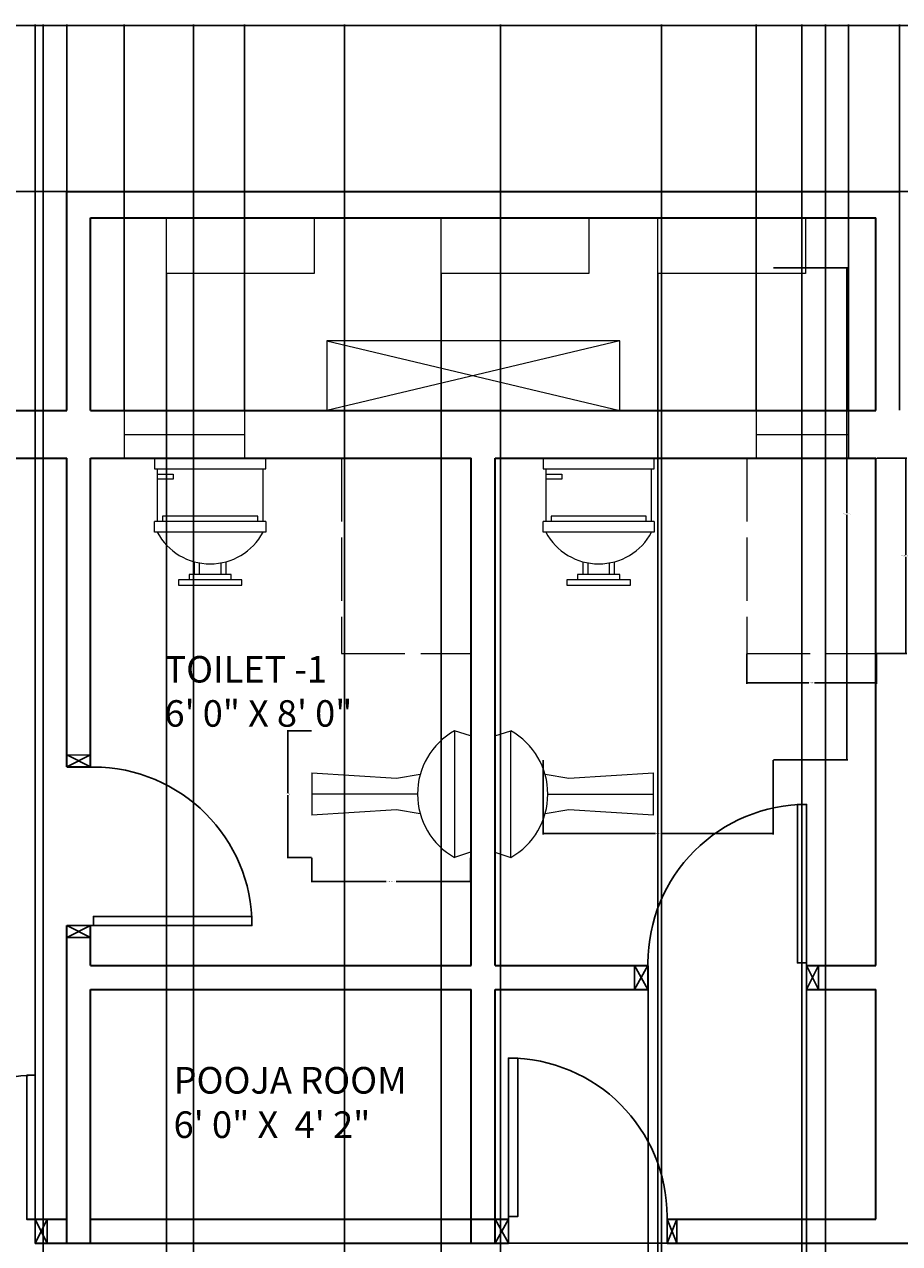
# Model space of a CAD drawing. Units: inches. Extents: x 2284228 to 3635239, y 3024422 to 8351872.
# Tile 6 of 7: x 3634888 to 3635054, y 8351600 to 8351831. Entities that reach past the tile are written whole.
import ezdxf

# ---------------------------------------------------------------- set-up
doc = ezdxf.new("R2010")
doc.units = ezdxf.units.IN
doc.linetypes.add('ACAD_ISO02W100', pattern=[15, 12, -3])
for name, color, linetype, lineweight in [('A-ANNO-DIMS', 2, 'Continuous', 18), ('A-AREA-IDEN', 7, 'Continuous', 18), ('A-DOOR', 4, 'Continuous', 25), ('A-EQPM', 8, 'Continuous', 18), ('A-FLOR-FIXT', 9, 'Continuous', 18), ('A-FLOR-FIXT-HIDN', 9, 'ACAD_ISO02W100', 18), ('A-GLAZ', 4, 'Continuous', 18), ('A-WALL', 7, 'Continuous', 35)]:
    doc.layers.add(name, color=color, linetype=linetype, lineweight=lineweight)
doc.styles.get("Standard").update_dxf_attribs({"font": 'arial.ttf'})
doc.dimstyles.get("Standard").update_dxf_attribs({"dimtxt": 0.18, "dimasz": 0.18, "dimexe": 0.18, "dimexo": 0.0625, "dimgap": 0.09, "dimtad": 0, "dimtih": 1, "dimtoh": 1, "dimdec": 4, "dimzin": 0, "dimdsep": 46, "dimtxsty": 'Standard', "dimcen": 0.09, "dimadec": 0, "dimazin": 0, "dimtfac": 1, "dimtdec": 4, "dimtofl": 0, "dimtmove": 0, "dimatfit": 3, "dimfxl": 1, "dimtolj": 1, "dimtzin": 0, "dimarcsym": 0})

# ---------------------------------------------------------------- blocks, each defined once
blk = doc.blocks.new('*U10')
for p, q in [((0, 0), (0, -5)), ((30, 0), (30, -5))]:
    blk.add_line(p, q)
blk.add_lwpolyline([(0, 0), (0, 30), (1.75, 30), (1.75, 0)], close=True)
blk.add_arc((0, 0), 30, 0, 90)
blk = doc.blocks.new('*U9')
for p, q in [((0, 0), (0, 5)), ((30, 0), (30, 5))]:
    blk.add_line(p, q)
blk.add_lwpolyline([(0, 0), (0, -30), (1.75, -30), (1.75, 0)], close=True)
blk.add_arc((0, 0), 30, 270, 0)
blk = doc.blocks.new('*U12')
for p, q in [((-30, 0), (-30, -5)), ((0, 0), (0, -5))]:
    blk.add_line(p, q)
blk.add_lwpolyline([(0, 0), (0, 30), (-1.75, 30), (-1.75, 0)], close=True)
blk.add_arc((0, 0), 30, 90, 180)
blk = doc.blocks.new('Toilet - Imperial')
for p, q in [((-10, 22), (-10, 12)), ((-10, 21), (-7, 21)), ((-7, 21), (-7, 20)), ((10, 12), (10, 22)), ((-7, 20), (-10, 20)), ((10.5, 12), (-10.5, 12)), ((-10.5, 10), (-10.5, 12)), ((9, 13), (-9, 13)), ((-9, 13), (-9, 12)), ((9, 12), (9, 13)), ((10.5, 12), (10.5, 10)), ((10.5, 10), (-10.5, 10)), ((-3, 4.4065), (-3, 2)), ((-2, 2), (-2, 4.1658)), ((2, 4.1658), (2, 2)), ((3, 2), (3, 4.4065)), ((4, 2), (-4, 2)), ((-4, 2), (-4, 1)), ((4, 1), (4, 2))]:
    blk.add_line(p, q)
for points in [[(10.5, 22), (10.5, 24), (-10.5, 24), (-10.5, 22)], [(6, 0), (6, 1), (-6, 1), (-6, 0)]]:
    blk.add_lwpolyline(points, close=True)
blk.add_arc((0, 15.3333), 11.3333, 208.0725, 331.9275)
blk = doc.blocks.new('Sink - Pedestal elevation')
for p, q in [((-11, 30), (-12, 27)), ((-11, 30), (11, 30)), ((11, 30), (12, 27)), ((-12, 27), (12, 27)), ((-3, 16), (-3.7523, 20.5139)), ((0, 20), (0, 0)), ((3.7527, 20.5157), (3, 16)), ((-4, 0), (-3, 16)), ((3, 16), (4, 0)), ((-4, 0), (4, 0))]:
    blk.add_line(p, q)
blk.add_arc((0, 33.7857), 13.7857, 209.4871, 330.5129)
blk = doc.blocks.new('SHOWER-OUTLINE')
for p, q in [((0, 36.97), (0, 0)), ((0, 0), (24.56, 0))]:
    blk.add_line(p, q)
blk = doc.blocks.new('SERVICE-LEDGE-MODULE')
blk.add_lwpolyline([(0, 10.53), (27.92, 10.53), (27.92, 0), (0, 0)], close=True)
blk = doc.blocks.new('*D32')
at = {"layer": 'A-ANNO-DIMS', "color": 0, "lineweight": -2, "transparency": 16777216}
for p, q in [((3635029.91, 8351784.56), (3635043.98, 8351784.56)), ((3635043.8, 8351784.38), (3635043.8, 8351738.22)), ((3635043.8, 8351691.7), (3635043.8, 8351737.86)), ((3635029.91, 8351691.52), (3635043.98, 8351691.52))]:
    blk.add_line(p, q, dxfattribs=at)
at = {"layer": 'A-ANNO-DIMS', "color": 0, "transparency": 16777216}
for points in [[(3635043.77, 8351784.38), (3635043.83, 8351784.38), (3635043.8, 8351784.56)], [(3635043.77, 8351691.7), (3635043.83, 8351691.7), (3635043.8, 8351691.52)]]:
    blk.add_solid(points, dxfattribs=at)
at = {"layer": 'Defpoints', "color": 0, "transparency": 16777216}
for p in [(3635029.85, 8351784.56), (3635043.8, 8351784.56), (3635029.85, 8351691.52)]:
    blk.add_point(p, dxfattribs=at)
at = {"layer": 'A-ANNO-DIMS', "color": 0, "transparency": 16777216, "insert": (3635043.8, 8351738.04), "char_height": 0.18, "attachment_point": 5}
blk.add_mtext('\\A1;WC 93 TYP.', dxfattribs=at)
blk = doc.blocks.new('*D33')
at = {"layer": 'A-ANNO-DIMS', "color": 0, "lineweight": -2, "transparency": 16777216}
for p, q in [((3634986.35, 8351691.45), (3634986.35, 8351677.38)), ((3635029.85, 8351691.45), (3635029.85, 8351677.38)), ((3634986.53, 8351677.56), (3635007.57, 8351677.56)), ((3635029.67, 8351677.56), (3635008.63, 8351677.56))]:
    blk.add_line(p, q, dxfattribs=at)
at = {"layer": 'A-ANNO-DIMS', "color": 0, "transparency": 16777216}
for points in [[(3634986.53, 8351677.59), (3634986.53, 8351677.53), (3634986.35, 8351677.56)], [(3635029.67, 8351677.59), (3635029.67, 8351677.53), (3635029.85, 8351677.56)]]:
    blk.add_solid(points, dxfattribs=at)
at = {"layer": 'Defpoints', "color": 0, "transparency": 16777216}
for p in [(3634986.35, 8351691.52), (3635029.85, 8351691.52), (3635029.85, 8351677.56)]:
    blk.add_point(p, dxfattribs=at)
at = {"layer": 'A-ANNO-DIMS', "color": 0, "transparency": 16777216, "insert": (3635008.1, 8351677.56), "char_height": 0.18, "attachment_point": 5}
blk.add_mtext('\\A1;44 TYP.', dxfattribs=at)
blk = doc.blocks.new('*D34')
at = {"layer": 'A-ANNO-DIMS', "color": 0, "lineweight": -2, "transparency": 16777216}
for p, q in [((3634942.58, 8351672.94), (3634942.58, 8351668.32)), ((3634972.58, 8351672.94), (3634972.58, 8351668.32)), ((3634942.76, 8351668.5), (3634956.64, 8351668.5)), ((3634972.4, 8351668.5), (3634958.51, 8351668.5))]:
    blk.add_line(p, q, dxfattribs=at)
at = {"layer": 'A-ANNO-DIMS', "color": 0, "transparency": 16777216}
for points in [[(3634942.76, 8351668.53), (3634942.76, 8351668.47), (3634942.58, 8351668.5)], [(3634972.4, 8351668.53), (3634972.4, 8351668.47), (3634972.58, 8351668.5)]]:
    blk.add_solid(points, dxfattribs=at)
at = {"layer": 'Defpoints', "color": 0, "transparency": 16777216}
for p in [(3634942.58, 8351673), (3634972.58, 8351673), (3634972.58, 8351668.5)]:
    blk.add_point(p, dxfattribs=at)
at = {"layer": 'A-ANNO-DIMS', "color": 0, "transparency": 16777216, "insert": (3634957.58, 8351668.5), "char_height": 0.18, "attachment_point": 5}
blk.add_mtext('\\A1;BASIN 30 TYP.', dxfattribs=at)
blk = doc.blocks.new('*D35')
at = {"layer": 'A-ANNO-DIMS', "color": 0, "lineweight": -2, "transparency": 16777216}
for p, q in [((3634942.51, 8351697), (3634937.9, 8351697)), ((3634938.08, 8351696.82), (3634938.08, 8351685.18)), ((3634938.08, 8351673.18), (3634938.08, 8351684.82)), ((3634942.51, 8351673), (3634937.9, 8351673))]:
    blk.add_line(p, q, dxfattribs=at)
at = {"layer": 'A-ANNO-DIMS', "color": 0, "transparency": 16777216}
for points in [[(3634938.05, 8351696.82), (3634938.11, 8351696.82), (3634938.08, 8351697)], [(3634938.05, 8351673.18), (3634938.11, 8351673.18), (3634938.08, 8351673)]]:
    blk.add_solid(points, dxfattribs=at)
at = {"layer": 'Defpoints', "color": 0, "transparency": 16777216}
for p in [(3634942.58, 8351697), (3634938.08, 8351673), (3634942.58, 8351673)]:
    blk.add_point(p, dxfattribs=at)
at = {"layer": 'A-ANNO-DIMS', "color": 0, "transparency": 16777216, "insert": (3634938.08, 8351685), "char_height": 0.18, "attachment_point": 5}
blk.add_mtext('\\A1;24 TYP.', dxfattribs=at)
blk = doc.blocks.new('*D38')
at = {"layer": 'A-ANNO-DIMS', "color": 0, "lineweight": -2, "transparency": 16777216}
for p, q in [((3635049.45, 8351748.56), (3635055.11, 8351748.56)), ((3635054.93, 8351748.38), (3635054.93, 8351730.26)), ((3635054.93, 8351711.77), (3635054.93, 8351729.89)), ((3635049.45, 8351711.59), (3635055.11, 8351711.59))]:
    blk.add_line(p, q, dxfattribs=at)
at = {"layer": 'A-ANNO-DIMS', "color": 0, "transparency": 16777216}
for points in [[(3635054.9, 8351748.38), (3635054.96, 8351748.38), (3635054.93, 8351748.56)], [(3635054.9, 8351711.77), (3635054.96, 8351711.77), (3635054.93, 8351711.59)]]:
    blk.add_solid(points, dxfattribs=at)
at = {"layer": 'Defpoints', "color": 0, "transparency": 16777216}
for p in [(3635049.39, 8351748.56), (3635054.93, 8351748.56), (3635049.39, 8351711.59)]:
    blk.add_point(p, dxfattribs=at)
at = {"layer": 'A-ANNO-DIMS', "color": 0, "transparency": 16777216, "insert": (3635054.93, 8351730.08), "char_height": 0.18, "attachment_point": 5}
blk.add_mtext('\\A1;SHOWER 37 TYP.', dxfattribs=at)
blk = doc.blocks.new('*D39')
at = {"layer": 'A-ANNO-DIMS', "color": 0, "lineweight": -2, "transparency": 16777216}
for p, q in [((3635024.83, 8351711.53), (3635024.83, 8351705.86)), ((3635049.39, 8351711.53), (3635049.39, 8351705.86)), ((3635025.01, 8351706.04), (3635036.58, 8351706.04)), ((3635049.21, 8351706.04), (3635037.64, 8351706.04))]:
    blk.add_line(p, q, dxfattribs=at)
at = {"layer": 'A-ANNO-DIMS', "color": 0, "transparency": 16777216}
for points in [[(3635025.01, 8351706.07), (3635025.01, 8351706.01), (3635024.83, 8351706.04)], [(3635049.21, 8351706.07), (3635049.21, 8351706.01), (3635049.39, 8351706.04)]]:
    blk.add_solid(points, dxfattribs=at)
at = {"layer": 'Defpoints', "color": 0, "transparency": 16777216}
for p in [(3635024.83, 8351711.59), (3635049.39, 8351711.59), (3635049.39, 8351706.04)]:
    blk.add_point(p, dxfattribs=at)
at = {"layer": 'A-ANNO-DIMS', "color": 0, "transparency": 16777216, "insert": (3635037.11, 8351706.04), "char_height": 0.18, "attachment_point": 5}
blk.add_mtext('\\A1;25 TYP.', dxfattribs=at)
blk = doc.blocks.new('*D41')
at = {"layer": 'A-ANNO-DIMS', "color": 0, "lineweight": -2, "transparency": 16777216}
for p, q in [((3635053.81, 8351799.01), (3635238.38, 8351799.01)), ((3635238.2, 8351798.83), (3635238.2, 8351524.72)), ((3635238.2, 8351250.24), (3635238.2, 8351524.36)), ((3635039.81, 8351250.06), (3635238.38, 8351250.06))]:
    blk.add_line(p, q, dxfattribs=at)
at = {"layer": 'A-ANNO-DIMS', "color": 0, "transparency": 16777216}
for points in [[(3635238.17, 8351798.83), (3635238.23, 8351798.83), (3635238.2, 8351799.01)], [(3635238.17, 8351250.24), (3635238.23, 8351250.24), (3635238.2, 8351250.06)]]:
    blk.add_solid(points, dxfattribs=at)
at = {"layer": 'Defpoints', "color": 0, "transparency": 16777216}
for p in [(3635053.75, 8351799.01), (3635238.2, 8351799.01), (3635039.75, 8351250.06)]:
    blk.add_point(p, dxfattribs=at)
at = {"layer": 'A-ANNO-DIMS', "color": 0, "transparency": 16777216, "insert": (3635238.2, 8351524.54), "char_height": 0.18, "attachment_point": 5}
blk.add_mtext('\\A1;549', dxfattribs=at)
blk = doc.blocks.new('*D42')
at = {"layer": 'A-ANNO-DIMS', "color": 0, "lineweight": -2, "transparency": 16777216}
for p, q in [((3634743.25, 8351757.63), (3634743.25, 8351830.64)), ((3634743.43, 8351830.46), (3634819.47, 8351830.46)), ((3634896.07, 8351830.46), (3634820.03, 8351830.46)), ((3634896.25, 8351757.63), (3634896.25, 8351830.64))]:
    blk.add_line(p, q, dxfattribs=at)
at = {"layer": 'A-ANNO-DIMS', "color": 0, "transparency": 16777216}
for points in [[(3634743.43, 8351830.49), (3634743.43, 8351830.43), (3634743.25, 8351830.46)], [(3634896.07, 8351830.49), (3634896.07, 8351830.43), (3634896.25, 8351830.46)]]:
    blk.add_solid(points, dxfattribs=at)
at = {"layer": 'Defpoints', "color": 0, "transparency": 16777216}
for p in [(3634896.25, 8351830.46), (3634743.25, 8351757.56), (3634896.25, 8351757.56)]:
    blk.add_point(p, dxfattribs=at)
at = {"layer": 'A-ANNO-DIMS', "color": 0, "transparency": 16777216, "insert": (3634819.75, 8351830.46), "char_height": 0.18, "attachment_point": 5}
blk.add_mtext('\\A1;153', dxfattribs=at)
blk = doc.blocks.new('*D43')
at = {"layer": 'A-ANNO-DIMS', "color": 0, "lineweight": -2, "transparency": 16777216}
for p, q in [((3634896.25, 8351799.07), (3634896.25, 8351830.64)), ((3634896.43, 8351830.46), (3634974.62, 8351830.46)), ((3635053.57, 8351830.46), (3634975.39, 8351830.46)), ((3635053.75, 8351799.07), (3635053.75, 8351830.64))]:
    blk.add_line(p, q, dxfattribs=at)
at = {"layer": 'A-ANNO-DIMS', "color": 0, "transparency": 16777216}
for points in [[(3634896.43, 8351830.49), (3634896.43, 8351830.43), (3634896.25, 8351830.46)], [(3635053.57, 8351830.49), (3635053.57, 8351830.43), (3635053.75, 8351830.46)]]:
    blk.add_solid(points, dxfattribs=at)
at = {"layer": 'Defpoints', "color": 0, "transparency": 16777216}
for p in [(3635053.75, 8351830.46), (3634896.25, 8351799.01), (3635053.75, 8351799.01)]:
    blk.add_point(p, dxfattribs=at)
at = {"layer": 'A-ANNO-DIMS', "color": 0, "transparency": 16777216, "insert": (3634975, 8351830.46), "char_height": 0.18, "attachment_point": 5}
blk.add_mtext('\\A1;157.5', dxfattribs=at)
blk = doc.blocks.new('*D44')
at = {"layer": 'A-ANNO-DIMS', "color": 0, "lineweight": -2, "transparency": 16777216}
for p, q in [((3635053.75, 8351757.63), (3635053.75, 8351830.64)), ((3635053.93, 8351830.46), (3635129.97, 8351830.46)), ((3635206.57, 8351830.46), (3635130.53, 8351830.46)), ((3635206.75, 8351757.63), (3635206.75, 8351830.64))]:
    blk.add_line(p, q, dxfattribs=at)
at = {"layer": 'A-ANNO-DIMS', "color": 0, "transparency": 16777216}
for points in [[(3635053.93, 8351830.49), (3635053.93, 8351830.43), (3635053.75, 8351830.46)], [(3635206.57, 8351830.49), (3635206.57, 8351830.43), (3635206.75, 8351830.46)]]:
    blk.add_solid(points, dxfattribs=at)
at = {"layer": 'Defpoints', "color": 0, "transparency": 16777216}
for p in [(3635206.75, 8351830.46), (3635053.75, 8351757.56), (3635206.75, 8351757.56)]:
    blk.add_point(p, dxfattribs=at)
at = {"layer": 'A-ANNO-DIMS', "color": 0, "transparency": 16777216, "insert": (3635130.25, 8351830.46), "char_height": 0.18, "attachment_point": 5}
blk.add_mtext('\\A1;153', dxfattribs=at)
blk = doc.blocks.new('*D45')
at = {"layer": 'A-ANNO-DIMS', "color": 0, "lineweight": -2, "transparency": 16777216}
for p, q in [((3634896.19, 8351799.01), (3634669.29, 8351799.01)), ((3634669.47, 8351798.83), (3634669.47, 8351778.47)), ((3634669.47, 8351757.74), (3634669.47, 8351778.11)), ((3634896.19, 8351757.56), (3634669.29, 8351757.56))]:
    blk.add_line(p, q, dxfattribs=at)
at = {"layer": 'A-ANNO-DIMS', "color": 0, "transparency": 16777216}
for points in [[(3634669.44, 8351798.83), (3634669.5, 8351798.83), (3634669.47, 8351799.01)], [(3634669.44, 8351757.74), (3634669.5, 8351757.74), (3634669.47, 8351757.56)]]:
    blk.add_solid(points, dxfattribs=at)
at = {"layer": 'Defpoints', "color": 0, "transparency": 16777216}
for p in [(3634669.47, 8351799.01), (3634896.25, 8351799.01), (3634896.25, 8351757.56)]:
    blk.add_point(p, dxfattribs=at)
at = {"layer": 'A-ANNO-DIMS', "color": 0, "transparency": 16777216, "insert": (3634669.47, 8351778.29), "char_height": 0.18, "attachment_point": 5}
blk.add_mtext('\\A1;41.45', dxfattribs=at)
blk = doc.blocks.new('*D49')
at = {"layer": 'A-ANNO-DIMS', "color": 0, "lineweight": -2, "transparency": 16777216}
for p, q in [((3634891.75, 8351310.63), (3634891.75, 8351830.64)), ((3634891.93, 8351830.46), (3634965.47, 8351830.46)), ((3635039.57, 8351830.46), (3634966.03, 8351830.46)), ((3635039.75, 8351310.63), (3635039.75, 8351830.64))]:
    blk.add_line(p, q, dxfattribs=at)
at = {"layer": 'A-ANNO-DIMS', "color": 0, "transparency": 16777216}
for points in [[(3634891.93, 8351830.49), (3634891.93, 8351830.43), (3634891.75, 8351830.46)], [(3635039.57, 8351830.49), (3635039.57, 8351830.43), (3635039.75, 8351830.46)]]:
    blk.add_solid(points, dxfattribs=at)
at = {"layer": 'Defpoints', "color": 0, "transparency": 16777216}
for p in [(3635039.75, 8351830.46), (3634891.75, 8351310.56), (3635039.75, 8351310.56)]:
    blk.add_point(p, dxfattribs=at)
at = {"layer": 'A-ANNO-DIMS', "color": 0, "transparency": 16777216, "insert": (3634965.75, 8351830.46), "char_height": 0.18, "attachment_point": 5}
blk.add_mtext('\\A1;148', dxfattribs=at)
blk = doc.blocks.new('*D54')
at = {"layer": 'A-ANNO-DIMS', "color": 0, "lineweight": -2, "transparency": 16777216}
for p, q in [((3635006.17, 8351652.5), (3635006.17, 8351218.43)), ((3635036.17, 8351652.5), (3635036.17, 8351218.43)), ((3635006.35, 8351218.61), (3635020.95, 8351218.61)), ((3635035.99, 8351218.61), (3635021.38, 8351218.61))]:
    blk.add_line(p, q, dxfattribs=at)
at = {"layer": 'A-ANNO-DIMS', "color": 0, "transparency": 16777216}
for points in [[(3635006.35, 8351218.64), (3635006.35, 8351218.58), (3635006.17, 8351218.61)], [(3635035.99, 8351218.64), (3635035.99, 8351218.58), (3635036.17, 8351218.61)]]:
    blk.add_solid(points, dxfattribs=at)
at = {"layer": 'Defpoints', "color": 0, "transparency": 16777216}
for p in [(3635006.17, 8351652.56), (3635036.17, 8351652.56), (3635036.17, 8351218.61)]:
    blk.add_point(p, dxfattribs=at)
at = {"layer": 'A-ANNO-DIMS', "color": 0, "transparency": 16777216, "insert": (3635021.17, 8351218.61), "char_height": 0.18, "attachment_point": 5}
blk.add_mtext('\\A1;30', dxfattribs=at)
blk = doc.blocks.new('*D55')
at = {"layer": 'A-ANNO-DIMS', "color": 0, "lineweight": -2, "transparency": 16777216}
for p, q in [((3634863.01, 8351604.61), (3634863.01, 8351830.64)), ((3634863.19, 8351830.46), (3634876.18, 8351830.46)), ((3634890.1, 8351830.46), (3634877.11, 8351830.46)), ((3634890.28, 8351604.61), (3634890.28, 8351830.64))]:
    blk.add_line(p, q, dxfattribs=at)
at = {"layer": 'A-ANNO-DIMS', "color": 0, "transparency": 16777216}
for points in [[(3634863.19, 8351830.49), (3634863.19, 8351830.43), (3634863.01, 8351830.46)], [(3634890.1, 8351830.49), (3634890.1, 8351830.43), (3634890.28, 8351830.46)]]:
    blk.add_solid(points, dxfattribs=at)
at = {"layer": 'Defpoints', "color": 0, "transparency": 16777216}
for p in [(3634890.28, 8351830.46), (3634863.01, 8351604.55), (3634890.28, 8351604.55)]:
    blk.add_point(p, dxfattribs=at)
at = {"layer": 'A-ANNO-DIMS', "color": 0, "transparency": 16777216, "insert": (3634876.64, 8351830.46), "char_height": 0.18, "attachment_point": 5}
blk.add_mtext('\\A1;27.265', dxfattribs=at)
blk = doc.blocks.new('*D57')
at = {"layer": 'A-ANNO-DIMS', "color": 0, "lineweight": -2, "transparency": 16777216}
for p, q in [((3635035.25, 8351378.63), (3635035.25, 8351830.64)), ((3635035.43, 8351830.46), (3635048.63, 8351830.46)), ((3635062.47, 8351830.46), (3635049.28, 8351830.46)), ((3635062.65, 8351378.63), (3635062.65, 8351830.64))]:
    blk.add_line(p, q, dxfattribs=at)
at = {"layer": 'A-ANNO-DIMS', "color": 0, "transparency": 16777216}
for points in [[(3635035.43, 8351830.49), (3635035.43, 8351830.43), (3635035.25, 8351830.46)], [(3635062.47, 8351830.49), (3635062.47, 8351830.43), (3635062.65, 8351830.46)]]:
    blk.add_solid(points, dxfattribs=at)
at = {"layer": 'Defpoints', "color": 0, "transparency": 16777216}
for p in [(3635062.65, 8351830.46), (3635035.25, 8351378.57), (3635062.65, 8351378.57)]:
    blk.add_point(p, dxfattribs=at)
at = {"layer": 'A-ANNO-DIMS', "color": 0, "transparency": 16777216, "insert": (3635048.95, 8351830.46), "char_height": 0.18, "attachment_point": 5}
blk.add_mtext('\\A1;27.4', dxfattribs=at)
blk = doc.blocks.new('*D67')
at = {"layer": 'A-ANNO-DIMS', "color": 0, "lineweight": -2, "transparency": 16777216}
for p, q in [((3634972.81, 8351600.06), (3635238.38, 8351600.06)), ((3635238.2, 8351599.88), (3635238.2, 8351588.44)), ((3635238.2, 8351576.63), (3635238.2, 8351588.08)), ((3634972.41, 8351576.45), (3635238.38, 8351576.45))]:
    blk.add_line(p, q, dxfattribs=at)
at = {"layer": 'A-ANNO-DIMS', "color": 0, "transparency": 16777216}
for points in [[(3635238.17, 8351599.88), (3635238.23, 8351599.88), (3635238.2, 8351600.06)], [(3635238.17, 8351576.63), (3635238.23, 8351576.63), (3635238.2, 8351576.45)]]:
    blk.add_solid(points, dxfattribs=at)
at = {"layer": 'Defpoints', "color": 0, "transparency": 16777216}
for p in [(3634972.75, 8351600.06), (3635238.2, 8351600.06), (3634972.35, 8351576.45)]:
    blk.add_point(p, dxfattribs=at)
at = {"layer": 'A-ANNO-DIMS', "color": 0, "transparency": 16777216, "insert": (3635238.2, 8351588.26), "char_height": 0.18, "attachment_point": 5}
blk.add_mtext('\\A1;23.61', dxfattribs=at)
blk = doc.blocks.new('*D72')
at = {"layer": 'A-ANNO-DIMS', "color": 0, "lineweight": -2, "transparency": 16777216}
for p, q in [((3634907.1, 8351757.63), (3634907.1, 8351830.64)), ((3634907.28, 8351830.46), (3634918.08, 8351830.46)), ((3634929.68, 8351830.46), (3634918.87, 8351830.46)), ((3634929.86, 8351757.63), (3634929.86, 8351830.64))]:
    blk.add_line(p, q, dxfattribs=at)
at = {"layer": 'A-ANNO-DIMS', "color": 0, "transparency": 16777216}
for points in [[(3634907.28, 8351830.49), (3634907.28, 8351830.43), (3634907.1, 8351830.46)], [(3634929.68, 8351830.49), (3634929.68, 8351830.43), (3634929.86, 8351830.46)]]:
    blk.add_solid(points, dxfattribs=at)
at = {"layer": 'Defpoints', "color": 0, "transparency": 16777216}
for p in [(3634929.86, 8351830.46), (3634907.1, 8351757.56), (3634929.86, 8351757.56)]:
    blk.add_point(p, dxfattribs=at)
at = {"layer": 'A-ANNO-DIMS', "color": 0, "transparency": 16777216, "insert": (3634918.48, 8351830.46), "char_height": 0.18, "attachment_point": 5}
blk.add_mtext('\\A1;22.76', dxfattribs=at)
blk = doc.blocks.new('*D73')
at = {"layer": 'A-ANNO-DIMS', "color": 0, "lineweight": -2, "transparency": 16777216}
for p, q in [((3635026.65107, 8351757.625221), (3635026.65107, 8351830.641759)), ((3635026.83107, 8351830.461759), (3635034.907727, 8351830.461759)), ((3635043.892856, 8351830.461759), (3635035.816199, 8351830.461759)), ((3635044.072856, 8351757.625221), (3635044.072856, 8351830.641759))]:
    blk.add_line(p, q, dxfattribs=at)
at = {"layer": 'A-ANNO-DIMS', "color": 0, "transparency": 16777216}
for points in [[(3635026.83107, 8351830.491759), (3635026.83107, 8351830.431759), (3635026.65107, 8351830.461759)], [(3635043.892856, 8351830.491759), (3635043.892856, 8351830.431759), (3635044.072856, 8351830.461759)]]:
    blk.add_solid(points, dxfattribs=at)
at = {"layer": 'Defpoints', "color": 0, "transparency": 16777216}
for p in [(3635044.072856, 8351830.461759), (3635026.65107, 8351757.562721), (3635044.072856, 8351757.562721)]:
    blk.add_point(p, dxfattribs=at)
at = {"layer": 'A-ANNO-DIMS', "color": 0, "transparency": 16777216, "insert": (3635035.361963, 8351830.461759), "char_height": 0.18, "attachment_point": 5}
blk.add_mtext('\\A1;17.422', dxfattribs=at)
blk = doc.blocks.new('*D74')
at = {"layer": 'A-ANNO-DIMS', "color": 0, "lineweight": -2, "transparency": 16777216}
for p, q in [((3634920.21, 8351331.63), (3634920.21, 8351830.64)), ((3634920.39, 8351830.46), (3634948.84, 8351830.46)), ((3634978.09, 8351830.46), (3634949.63, 8351830.46)), ((3634978.27, 8351331.63), (3634978.27, 8351830.64))]:
    blk.add_line(p, q, dxfattribs=at)
at = {"layer": 'A-ANNO-DIMS', "color": 0, "transparency": 16777216}
for points in [[(3634920.39, 8351830.49), (3634920.39, 8351830.43), (3634920.21, 8351830.46)], [(3634978.09, 8351830.49), (3634978.09, 8351830.43), (3634978.27, 8351830.46)]]:
    blk.add_solid(points, dxfattribs=at)
at = {"layer": 'Defpoints', "color": 0, "transparency": 16777216}
for p in [(3634978.27, 8351830.46), (3634920.21, 8351331.56), (3634978.27, 8351331.56)]:
    blk.add_point(p, dxfattribs=at)
at = {"layer": 'A-ANNO-DIMS', "color": 0, "transparency": 16777216, "insert": (3634949.24, 8351830.46), "char_height": 0.18, "attachment_point": 5}
blk.add_mtext('\\A1;58.06', dxfattribs=at)
blk = doc.blocks.new('*D80')
at = {"layer": 'A-ANNO-DIMS', "color": 0, "lineweight": -2, "transparency": 16777216}
for p, q in [((3634948.75, 8351437.56), (3634948.75, 8351830.64)), ((3634948.93, 8351830.46), (3634978.53, 8351830.46)), ((3635008.57, 8351830.46), (3634978.97, 8351830.46)), ((3635008.75, 8351437.56), (3635008.75, 8351830.64))]:
    blk.add_line(p, q, dxfattribs=at)
at = {"layer": 'A-ANNO-DIMS', "color": 0, "transparency": 16777216}
for points in [[(3634948.93, 8351830.49), (3634948.93, 8351830.43), (3634948.75, 8351830.46)], [(3635008.57, 8351830.49), (3635008.57, 8351830.43), (3635008.75, 8351830.46)]]:
    blk.add_solid(points, dxfattribs=at)
at = {"layer": 'Defpoints', "color": 0, "transparency": 16777216}
for p in [(3635008.75, 8351830.46), (3634948.75, 8351437.49), (3635008.75, 8351437.49)]:
    blk.add_point(p, dxfattribs=at)
at = {"layer": 'A-ANNO-DIMS', "color": 0, "transparency": 16777216, "insert": (3634978.75, 8351830.46), "char_height": 0.18, "attachment_point": 5}
blk.add_mtext('\\A1;60', dxfattribs=at)
blk = doc.blocks.new('*D82')
at = {"layer": 'A-ANNO-DIMS', "color": 0, "lineweight": -2, "transparency": 16777216}
for p, q in [((3634915.11, 8351783.43), (3634915.11, 8351218.43)), ((3634967.04, 8351783.43), (3634967.04, 8351218.43)), ((3634915.29, 8351218.61), (3634940.68, 8351218.61)), ((3634966.86, 8351218.61), (3634941.47, 8351218.61))]:
    blk.add_line(p, q, dxfattribs=at)
at = {"layer": 'A-ANNO-DIMS', "color": 0, "transparency": 16777216}
for points in [[(3634915.29, 8351218.64), (3634915.29, 8351218.58), (3634915.11, 8351218.61)], [(3634966.86, 8351218.64), (3634966.86, 8351218.58), (3634967.04, 8351218.61)]]:
    blk.add_solid(points, dxfattribs=at)
at = {"layer": 'Defpoints', "color": 0, "transparency": 16777216}
for p in [(3634915.11, 8351783.5), (3634967.04, 8351783.5), (3634967.04, 8351218.61)]:
    blk.add_point(p, dxfattribs=at)
at = {"layer": 'A-ANNO-DIMS', "color": 0, "transparency": 16777216, "insert": (3634941.08, 8351218.61), "char_height": 0.18, "attachment_point": 5}
blk.add_mtext('\\A1;51.94', dxfattribs=at)
blk = doc.blocks.new('*D83')
at = {"layer": 'A-ANNO-DIMS', "color": 0, "lineweight": -2, "transparency": 16777216}
for p, q in [((3634967.04, 8351783.43), (3634967.04, 8351218.43)), ((3635008.03, 8351783.43), (3635008.03, 8351218.43)), ((3634967.22, 8351218.61), (3634987.14, 8351218.61)), ((3635007.85, 8351218.61), (3634987.93, 8351218.61))]:
    blk.add_line(p, q, dxfattribs=at)
at = {"layer": 'A-ANNO-DIMS', "color": 0, "transparency": 16777216}
for points in [[(3634967.22, 8351218.64), (3634967.22, 8351218.58), (3634967.04, 8351218.61)], [(3635007.85, 8351218.64), (3635007.85, 8351218.58), (3635008.03, 8351218.61)]]:
    blk.add_solid(points, dxfattribs=at)
at = {"layer": 'Defpoints', "color": 0, "transparency": 16777216}
for p in [(3634967.04, 8351783.5), (3635008.03, 8351783.5), (3635008.03, 8351218.61)]:
    blk.add_point(p, dxfattribs=at)
at = {"layer": 'A-ANNO-DIMS', "color": 0, "transparency": 16777216, "insert": (3634987.54, 8351218.61), "char_height": 0.18, "attachment_point": 5}
blk.add_mtext('\\A1;40.98', dxfattribs=at)

msp = doc.modelspace()

# ---------------------------------------------------------------- linework, layer by layer
at = {"layer": 'A-DOOR'}
for p, q in [((3634896.2379, 8351690.1408), (3634900.7379, 8351692.4094)), ((3634896.2379, 8351692.4094), (3634900.7379, 8351690.1408)), ((3634896.2525, 8351692.4021), (3634900.7379, 8351692.4094)), ((3634900.7379, 8351690.1408), (3634896.2379, 8351690.1408)), ((3634896.2525, 8351657.8523), (3634900.7525, 8351660.121)), ((3634896.2525, 8351660.121), (3634900.7525, 8351657.8523)), ((3634900.7525, 8351657.8523), (3634896.2525, 8351657.8523)), ((3635006.1658, 8351652.5627), (3635003.594, 8351652.5627)), ((3635003.594, 8351652.5627), (3635003.594, 8351648.0627)), ((3635003.594, 8351652.5627), (3635006.1658, 8351648.0627)), ((3635003.594, 8351648.0627), (3635006.1658, 8351652.5627)), ((3635036.1658, 8351652.5627), (3635038.4172, 8351652.5627)), ((3635036.1658, 8351652.5627), (3635038.4172, 8351648.0627)), ((3635036.1658, 8351648.0627), (3635038.4172, 8351652.5627)), ((3635038.4172, 8351652.5627), (3635038.4172, 8351648.0627)), ((3634892.5451, 8351600.0487), (3634890.2764, 8351604.5487)), ((3634890.2764, 8351600.0487), (3634892.5451, 8351604.5487)), ((3634890.2764, 8351600.0487), (3634890.2764, 8351604.5487)), ((3634892.5451, 8351604.5487), (3634892.5451, 8351600.0487)), ((3634977.2525, 8351604.5627), (3634979.7751, 8351604.5627)), ((3634977.2525, 8351604.5627), (3634979.7751, 8351600.0627)), ((3634977.2525, 8351600.0627), (3634979.7751, 8351604.5627)), ((3634979.7751, 8351604.5627), (3634979.7751, 8351600.0627)), ((3635009.7751, 8351604.5627), (3635011.6318, 8351604.5627)), ((3635009.7751, 8351604.5627), (3635011.6318, 8351600.0627)), ((3635009.7751, 8351600.0566), (3635011.6318, 8351604.5627)), ((3635011.6318, 8351604.5627), (3635011.6318, 8351600.0627))]:
    msp.add_line(p, q, dxfattribs=at)
at = {"layer": 'A-EQPM'}
for p, q in [((3634945.4201, 8351770.7868), (3635000.8245, 8351757.5627)), ((3635000.8245, 8351770.7868), (3634945.4201, 8351757.5627))]:
    msp.add_line(p, q, dxfattribs=at)
msp.add_lwpolyline([(3634945.4201, 8351757.5627), (3635000.8245, 8351757.5627), (3635000.8245, 8351770.7868), (3634945.4201, 8351770.7868)], close=True, dxfattribs=at)
at = {"layer": 'A-GLAZ'}
for p, q in [((3634907.0987, 8351757.5627), (3634907.0987, 8351748.5627)), ((3634907.0987, 8351757.5627), (3634929.8577, 8351757.5627)), ((3634929.8577, 8351757.5627), (3634929.8577, 8351748.5627)), ((3635026.6511, 8351757.5627), (3635026.6511, 8351748.5627)), ((3635044.0729, 8351757.5627), (3635044.0729, 8351748.5627)), ((3634907.0987, 8351753.0627), (3634929.8577, 8351753.0627)), ((3635026.6511, 8351753.0627), (3635044.0729, 8351753.0627))]:
    msp.add_line(p, q, dxfattribs=at)
at = {"layer": 'A-WALL'}
for p, q in [((3634896.2525, 8351799.0118), (3635053.7525, 8351799.0118)), ((3634896.2525, 8351757.5627), (3634896.2525, 8351799.0118)), ((3634900.7525, 8351794.031), (3635049.2525, 8351794.031)), ((3634900.7525, 8351757.5627), (3634900.7525, 8351794.031)), ((3635049.2525, 8351757.5627), (3635049.2525, 8351794.031)), ((3634743.2525, 8351757.5627), (3634896.2525, 8351757.5627)), ((3634900.7525, 8351757.5627), (3635049.2525, 8351757.5627)), ((3634852.7525, 8351748.5627), (3634896.2525, 8351748.5627)), ((3634896.2525, 8351690.1408), (3634896.2525, 8351748.5627)), ((3634896.2525, 8351690.1408), (3634896.2525, 8351748.5627)), ((3634900.7525, 8351748.5627), (3634972.7525, 8351748.5627)), ((3634900.7525, 8351690.121), (3634900.7525, 8351748.5627)), ((3634900.7525, 8351690.121), (3634900.7525, 8351748.5627)), ((3634972.7525, 8351652.5627), (3634972.7525, 8351748.5627)), ((3634977.2525, 8351652.5627), (3634977.2525, 8351748.5627)), ((3634977.2525, 8351748.5627), (3635049.2525, 8351748.5627)), ((3635049.2525, 8351652.5627), (3635049.2525, 8351748.5627)), ((3634896.2525, 8351600.0627), (3634896.2525, 8351660.121)), ((3634896.2525, 8351604.5627), (3634896.2525, 8351660.121)), ((3634900.7525, 8351652.5627), (3634900.7525, 8351660.121)), ((3634900.7525, 8351652.5627), (3634900.7525, 8351660.121)), ((3634900.7525, 8351652.5627), (3634972.7525, 8351652.5627)), ((3634900.7525, 8351652.5627), (3634972.7525, 8351652.5627)), ((3634977.2525, 8351652.5627), (3635006.1658, 8351652.5627)), ((3634977.2525, 8351652.5627), (3635006.1658, 8351652.5627)), ((3635036.1658, 8351652.5627), (3635049.2525, 8351652.5627)), ((3635036.1658, 8351652.5627), (3635049.2525, 8351652.5627)), ((3634900.7525, 8351648.0627), (3634972.7525, 8351648.0627)), ((3634900.7525, 8351600.0627), (3634900.7525, 8351648.0627)), ((3634900.7525, 8351604.5627), (3634900.7525, 8351648.0627)), ((3634972.7525, 8351600.0627), (3634972.7525, 8351648.0627)), ((3634977.2525, 8351600.0627), (3634977.2525, 8351648.0627)), ((3634977.2525, 8351648.0627), (3635006.1658, 8351648.0627)), ((3635036.1658, 8351648.0627), (3635049.2525, 8351648.0627)), ((3635049.2525, 8351604.5627), (3635049.2525, 8351648.0627)), ((3634888.686, 8351604.5627), (3634896.2525, 8351604.5627)), ((3634888.686, 8351604.5627), (3634896.2525, 8351604.5627)), ((3634900.7525, 8351604.5627), (3634972.7525, 8351604.5627)), ((3634900.7525, 8351604.5627), (3634979.7751, 8351604.5627)), ((3634977.2525, 8351604.5627), (3634979.7751, 8351604.5627)), ((3635009.7751, 8351604.5627), (3635049.2525, 8351604.5627)), ((3635009.7751, 8351604.5627), (3635049.2525, 8351604.5627)), ((3634890.2764, 8351600.0627), (3634896.2525, 8351600.0627)), ((3634896.2525, 8351600.0627), (3634979.7751, 8351600.0627)), ((3635009.7751, 8351600.0627), (3635197.7525, 8351600.0627))]:
    msp.add_line(p, q, dxfattribs=at)

# ---------------------------------------------------------------- block references
at = {"layer": 'A-DOOR'}
for name, p, rotation in [('*U12', (3634901.2751, 8351660.121), 270), ('*U9', (3635036.1658, 8351653.0517), 180)]:
    msp.add_blockref(name, p, dxfattribs=dict(at, rotation=rotation))
msp.add_blockref('*U10', (3634979.7751, 8351605.0566), dxfattribs=at)
at = {"layer": 'A-DOOR', "xscale": 0.9088208868574007, "yscale": 0.9088208868574007, "zscale": 0.9088208868574007, "rotation": 180}
msp.add_blockref('*U9', (3634890.2764, 8351604.5487), dxfattribs=at)
at = {"layer": 'A-EQPM'}
for p in [(3634915.106, 8351783.497), (3634967.045, 8351783.497), (3635008.0261, 8351783.497)]:
    msp.add_blockref('SERVICE-LEDGE-MODULE', p, dxfattribs=at)
at = {"layer": 'A-FLOR-FIXT'}
for p in [(3634923.3612, 8351724.5627), (3634996.8471, 8351724.5627)]:
    msp.add_blockref('Toilet - Imperial', p, dxfattribs=at)
for p, rotation in [((3634942.5774, 8351685.0022), 270), ((3635007.2194, 8351685.0022), 89.99999999999999)]:
    msp.add_blockref('Sink - Pedestal elevation', p, dxfattribs=dict(at, rotation=rotation))
at = {"layer": 'A-FLOR-FIXT-HIDN'}
for p in [(3634948.195, 8351711.589), (3635024.8293, 8351711.589)]:
    msp.add_blockref('SHOWER-OUTLINE', p, dxfattribs=at)

# ---------------------------------------------------------------- texts
at = {"layer": 'A-AREA-IDEN', "attachment_point": 1}
for s, width, gutter_width, insert, char_height in [('    TOILET -1\\P    6\' 0" X 8\' 0"', 251.703932, 25.0736, (3634908.6006, 8351711.133), 5.014726), ('    POOJA ROOM \\P    6\' 0" X  4\' 2"', 142.396495, 25.1871, (3634910.2789, 8351633.3764), 5.037427)]:
    msp.add_mtext_dynamic_manual_height_columns(s, width=width, gutter_width=gutter_width, heights=[0], dxfattribs=dict(at, insert=insert, char_height=char_height))

# ---------------------------------------------------------------- dimensions: what is measured, and where the dimension line sits
at = {"layer": 'A-ANNO-DIMS'}
for base, p1, p2, override, picture, middle in [((3634896.2525, 8351830.4618), (3634743.2525, 8351757.5627), (3634896.2525, 8351757.5627), {"dimdec": 0, "dimlfac": 1, "dimrnd": 0, "dimzin": 0, "dimdsep": 46, "dimlunit": 2}, '*D42', (3634819.7525, 8351830.4618)), ((3634890.2764, 8351830.4618), (3634863.0118, 8351604.5487), (3634890.2764, 8351604.5487), {"dimdec": 3, "dimlfac": 1, "dimrnd": 0, "dimzin": 0, "dimdsep": 46, "dimlunit": 2}, '*D55', (3634876.6441, 8351830.4618)), ((3635039.7525, 8351830.4618), (3634891.7525, 8351310.5627), (3635039.7525, 8351310.5627), {"dimdec": 0, "dimlfac": 1, "dimrnd": 0, "dimzin": 0, "dimdsep": 46, "dimlunit": 2}, '*D49', (3634965.7525, 8351830.4618)), ((3635053.7525, 8351830.4618), (3634896.2525, 8351799.0118), (3635053.7525, 8351799.0118), {"dimdec": 1, "dimlfac": 1, "dimrnd": 0, "dimzin": 0, "dimdsep": 46, "dimlunit": 2}, '*D43', (3634975.0025, 8351830.4618)), ((3634929.8577, 8351830.4618), (3634907.0987, 8351757.5627), (3634929.8577, 8351757.5627), {"dimdec": 2, "dimlfac": 1, "dimrnd": 0, "dimzin": 0, "dimdsep": 46, "dimlunit": 2}, '*D72', (3634918.4782, 8351830.4618)), ((3634978.266, 8351830.4618), (3634920.2105, 8351331.5627), (3634978.266, 8351331.5627), {"dimdec": 2, "dimlfac": 1, "dimrnd": 0, "dimzin": 0, "dimdsep": 46, "dimlunit": 2}, '*D74', (3634949.2383, 8351830.4618)), ((3635008.7462, 8351830.4618), (3634948.7462, 8351437.4931), (3635008.7462, 8351437.4931), {"dimdec": 0, "dimlfac": 1, "dimrnd": 0, "dimzin": 0, "dimdsep": 46, "dimlunit": 2}, '*D80', (3634978.7462, 8351830.4618)), ((3635044.0729, 8351830.4618), (3635026.6511, 8351757.5627), (3635044.0729, 8351757.5627), {"dimdec": 3, "dimlfac": 1, "dimrnd": 0, "dimzin": 0, "dimdsep": 46, "dimlunit": 2}, '*D73', (3635035.362, 8351830.4618)), ((3635062.6524, 8351830.4618), (3635035.2525, 8351378.5661), (3635062.6524, 8351378.5661), {"dimdec": 1, "dimlfac": 1, "dimrnd": 0, "dimzin": 0, "dimdsep": 46, "dimlunit": 2}, '*D57', (3635048.9524, 8351830.4618)), ((3635206.7525, 8351830.4618), (3635053.7525, 8351757.5627), (3635206.7525, 8351757.5627), {"dimdec": 0, "dimlfac": 1, "dimrnd": 0, "dimzin": 0, "dimdsep": 46, "dimlunit": 2}, '*D44', (3635130.2525, 8351830.4618)), ((3634967.0447, 8351218.6127), (3634915.1056, 8351783.4971), (3634967.0447, 8351783.4971), {"dimdec": 2, "dimlfac": 1, "dimrnd": 0, "dimzin": 0, "dimdsep": 46, "dimlunit": 2}, '*D82', (3634941.0752, 8351218.6127)), ((3635008.0257, 8351218.6127), (3634967.0447, 8351783.4971), (3635008.0257, 8351783.4971), {"dimdec": 2, "dimlfac": 1, "dimrnd": 0, "dimzin": 0, "dimdsep": 46, "dimlunit": 2}, '*D83', (3634987.5352, 8351218.6127)), ((3635036.1658, 8351218.6127), (3635006.1658, 8351652.5627), (3635036.1658, 8351652.5627), {"dimdec": 0, "dimlfac": 1, "dimrnd": 0, "dimzin": 0, "dimdsep": 46, "dimlunit": 2}, '*D54', (3635021.1658, 8351218.6127))]:
    dim = msp.add_linear_dim(base=base, p1=p1, p2=p2, dimstyle='Standard', override=override, dxfattribs=at)
    dim.commit()
    dim.dimension.update_dxf_attribs({"geometry": picture, "text_midpoint": middle})
for base, p1, p2, override, picture, middle in [((3634669.465, 8351799.0118), (3634896.2525, 8351757.5627), (3634896.2525, 8351799.0118), {"dimdec": 2, "dimlfac": 1, "dimrnd": 0, "dimzin": 0, "dimdsep": 46, "dimlunit": 2}, '*D45', (3634669.465, 8351778.2872)), ((3635238.2025, 8351799.0118), (3635039.7525, 8351250.0627), (3635053.7525, 8351799.0118), {"dimdec": 0, "dimlfac": 1, "dimrnd": 0, "dimzin": 0, "dimdsep": 46, "dimlunit": 2}, '*D41', (3635238.2025, 8351524.5372)), ((3635238.2025, 8351600.0627), (3634972.3485, 8351576.4517), (3634972.7525, 8351600.0627), {"dimdec": 2, "dimlfac": 1, "dimrnd": 0, "dimzin": 0, "dimdsep": 46, "dimlunit": 2}, '*D67', (3635238.2025, 8351588.2572))]:
    dim = msp.add_linear_dim(base=base, p1=p1, p2=p2, angle=90, dimstyle='Standard', override=override, dxfattribs=at)
    dim.commit()
    dim.dimension.update_dxf_attribs({"geometry": picture, "text_midpoint": middle})
for base, p1, p2, angle, text, picture, middle in [((3635043.804, 8351784.5627), (3635029.8471, 8351691.5165), (3635029.8471, 8351784.5627), 90, 'WC <> TYP.', '*D32', (3635043.804, 8351738.0396)), ((3635054.9328, 8351748.5627), (3635049.3867, 8351711.5887), (3635049.3867, 8351748.5627), 90, 'SHOWER <> TYP.', '*D38', (3635054.9328, 8351730.0757)), ((3634938.0774, 8351673.0022), (3634942.5774, 8351697.0022), (3634942.5774, 8351673.0022), 270, '<> TYP.', '*D35', (3634938.0774, 8351685.0022))]:
    dim = msp.add_linear_dim(base=base, p1=p1, p2=p2, angle=angle, text=text, dimstyle='Standard', override={"dimdec": 0, "dimlfac": 1, "dimrnd": 0, "dimzin": 0, "dimdsep": 46, "dimlunit": 2}, dxfattribs=at)
    dim.commit()
    dim.dimension.update_dxf_attribs({"geometry": picture, "text_midpoint": middle})
for base, p1, p2, text, picture, middle in [((3635049.3867, 8351706.0426), (3635024.829, 8351711.5887), (3635049.3867, 8351711.5887), '<> TYP.', '*D39', (3635037.1079, 8351706.0426)), ((3635029.8470890522, 8351677.5595399523), (3634986.3470890522, 8351691.5164765753), (3635029.8470890522, 8351691.5164765753), '<> TYP.', '*D33', (3635008.0970890522, 8351677.5595399523)), ((3634972.5774, 8351668.5022), (3634942.5774, 8351673.0022), (3634972.5774, 8351673.0022), 'BASIN <> TYP.', '*D34', (3634957.5774, 8351668.5022))]:
    dim = msp.add_linear_dim(base=base, p1=p1, p2=p2, text=text, dimstyle='Standard', override={"dimdec": 0, "dimlfac": 1, "dimrnd": 0, "dimzin": 0, "dimdsep": 46, "dimlunit": 2}, dxfattribs=at)
    dim.commit()
    dim.dimension.update_dxf_attribs({"geometry": picture, "text_midpoint": middle})

doc.saveas('drawing.dxf')
